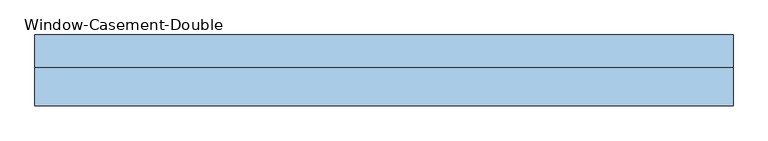
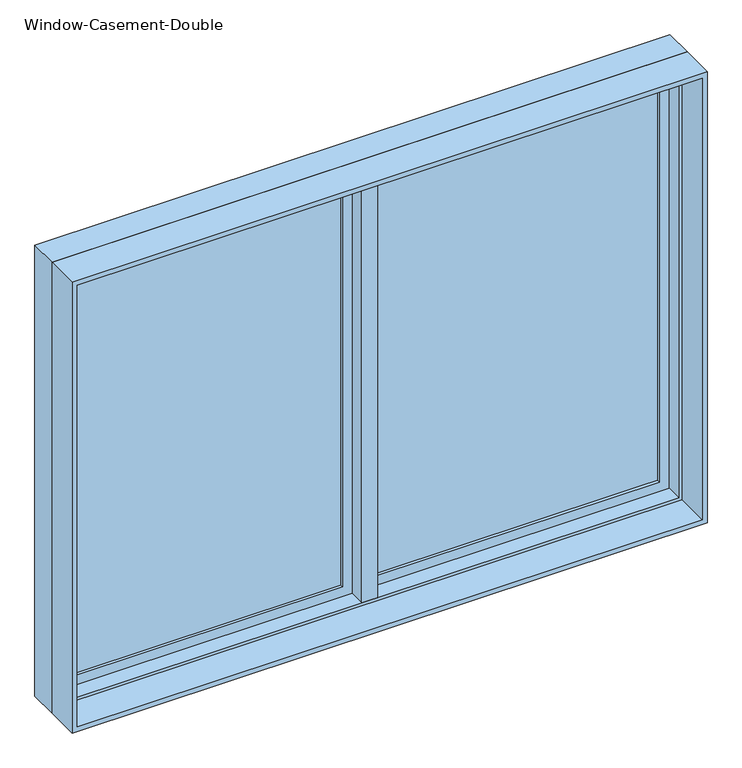
"""IFC4 building model written with IfcOpenShell, lengths in millimetres: window geometry, Window-Casement-Double."""

from ifc_helpers import new_model, si_unit, frame, origin, place, context, project, spatial, polyline, outline, extrude, faceted_brep, source, transform, mapped, element, save


def window_casement_double_9ae172a2(model_context):
    return source(origin(), model_context, "Body", "SolidModel", [
        faceted_brep([(9.525, 133.35, 2730.5), (-9.525, 133.35, 2730.5), (-9.525, 82.55, 2730.5), (9.525, 82.55, 2730.5), (9.525, 133.35, 927.1), (9.525, 82.55, 927.1), (-9.525, 82.55, 927.1), (-9.525, 133.35, 927.1), (-9.525, 82.55, 946.15), (-9.525, 82.55, 2711.45), (-30.1625, 82.55, 946.15), (-30.1625, 82.55, 2711.45), (-30.1625, 19.05, 946.15), (-30.1625, 19.05, 2711.45), (30.1625, 19.05, 946.15), (30.1625, 19.05, 2711.45), (30.1625, 82.55, 946.15), (30.1625, 82.55, 2711.45), (9.525, 82.55, 946.15), (9.525, 82.55, 2711.45)], [[[0, 1, 2, 3]], [[4, 5, 6, 7]], [[1, 0, 4, 7]], [[2, 1, 7, 6, 8, 9]], [[9, 8, 10, 11]], [[11, 10, 12, 13]], [[13, 12, 14, 15]], [[15, 14, 16, 17]], [[17, 16, 18, 19]], [[0, 3, 19, 18, 5, 4]], [[18, 8, 6, 5]], [[9, 19, 3, 2]], [[8, 18, 16, 14, 12, 10]], [[19, 9, 11, 13, 15, 17]]]),
        extrude(outline(polyline([(-66.675, 114.3), (-66.675, 107.95), (-1149.35, 107.95), (-1149.35, 114.3), (-66.675, 114.3)])), frame((0.0, 0.0, 984.25), z_axis=(0.0, 0.0, 1.0), x_axis=(1.0, 0.0, 0.0)), (0.0, 0.0, 1.0), 1689.1),
        extrude(outline(polyline([(-1149.35, 95.25), (-1149.35, 101.6), (-66.675, 101.6), (-66.675, 95.25), (-1149.35, 95.25)])), frame((0.0, 0.0, 984.25), z_axis=(0.0, 0.0, 1.0), x_axis=(1.0, 0.0, 0.0)), (0.0, 0.0, 1.0), 1689.1),
        extrude(outline(polyline([(1149.35, 114.3), (1149.35, 107.95), (66.675, 107.95), (66.675, 114.3), (1149.35, 114.3)])), frame((0.0, 0.0, 984.25), z_axis=(0.0, 0.0, 1.0), x_axis=(1.0, 0.0, 0.0)), (0.0, 0.0, 1.0), 1689.1),
        extrude(outline(polyline([(66.675, 95.25), (66.675, 101.6), (1149.35, 101.6), (1149.35, 95.25), (66.675, 95.25)])), frame((0.0, 0.0, 984.25), z_axis=(0.0, 0.0, 1.0), x_axis=(1.0, 0.0, 0.0)), (0.0, 0.0, 1.0), 1689.1),
        extrude(outline(polyline([(2730.5, -1206.5), (927.1, -1206.5), (927.1, -9.525), (2730.5, -9.525), (2730.5, -1206.5)]), holes=[polyline([(2673.35, -66.675), (984.25, -66.675), (984.25, -1149.35), (2673.35, -1149.35), (2673.35, -66.675)])]), frame((0.0, 82.55, 0.0), z_axis=(0.0, 1.0, 0.0), x_axis=(0.0, 0.0, 1.0)), (0.0, 0.0, 1.0), 44.45),
        extrude(outline(polyline([(927.1, 1206.5), (2730.5, 1206.5), (2730.5, 9.525), (927.1, 9.525), (927.1, 1206.5)]), holes=[polyline([(984.25, 66.675), (2673.35, 66.675), (2673.35, 1149.35), (984.25, 1149.35), (984.25, 66.675)])]), frame((0.0, 82.55, 0.0), z_axis=(0.0, 1.0, 0.0), x_axis=(0.0, 0.0, 1.0)), (0.0, 0.0, 1.0), 44.45),
        extrude(outline(polyline([(2743.2, -1219.2), (914.4, -1219.2), (914.4, 1219.2), (2743.2, 1219.2), (2743.2, -1219.2)]), holes=[polyline([(2724.15, 1200.15), (933.45, 1200.15), (933.45, -1200.15), (2724.15, -1200.15), (2724.15, 1200.15)])]), frame((0.0, -114.3, 0.0), z_axis=(0.0, 1.0, 0.0), x_axis=(0.0, 0.0, 1.0)), (0.0, 0.0, 1.0), 133.35),
        faceted_brep([(1187.45, 82.55, 2711.45), (1187.45, 19.05, 2711.45), (-1187.45, 19.05, 2711.45), (-1187.45, 82.55, 2711.45), (1206.5, 133.35, 2730.5), (1206.5, 82.55, 2730.5), (-1206.5, 82.55, 2730.5), (-1206.5, 133.35, 2730.5), (1219.2, 19.05, 2743.2), (1219.2, 133.35, 2743.2), (-1219.2, 133.35, 2743.2), (-1219.2, 19.05, 2743.2), (-1187.45, 19.05, 946.15), (-1187.45, 82.55, 946.15), (-1206.5, 82.55, 927.1), (-1206.5, 133.35, 927.1), (-1219.2, 133.35, 914.4), (-1219.2, 19.05, 914.4), (1187.45, 19.05, 946.15), (1187.45, 82.55, 946.15), (1206.5, 82.55, 927.1), (1206.5, 133.35, 927.1), (1219.2, 133.35, 914.4), (1219.2, 19.05, 914.4)], [[[0, 1, 2, 3]], [[4, 5, 6, 7]], [[8, 9, 10, 11]], [[3, 2, 12, 13]], [[7, 6, 14, 15]], [[11, 10, 16, 17]], [[13, 12, 18, 19]], [[15, 14, 20, 21]], [[17, 16, 22, 23]], [[11, 17, 23, 8], [1, 18, 12, 2]], [[19, 18, 1, 0]], [[5, 20, 14, 6], [3, 13, 19, 0]], [[21, 20, 5, 4]], [[23, 22, 9, 8]], [[9, 22, 16, 10], [7, 15, 21, 4]]]),
    ])


if __name__ == "__main__":
    model = new_model("IFC4")
    model_context = context("Model", 3, world=origin())
    ifc_project = project(units=[si_unit("LENGTHUNIT", "METRE", prefix="MILLI")], contexts=[model_context])
    site = spatial("IfcSite", under=ifc_project)
    building = spatial("IfcBuilding", under=site)
    placement = place(None, origin())
    window_casement_double_shape = window_casement_double_9ae172a2(model_context)
    element("IfcWindow", 1, ObjectType="Window-Casement-Double", at=placement, inside=building, context=model_context, shape_type="MappedRepresentation", body=[
        mapped(window_casement_double_shape, transform((0.0, 0.0, 0.0), x_axis=(1.0, 0.0, 0.0), y_axis=(0.0, 1.0, 0.0), z_axis=(0.0, 0.0, 1.0))),
    ])
    save(model, "model.ifc")

# Revit data of these elements
# Type "Window-Casement-Double"
#   Type Mark = "19"
#   Fire Rating = "0.5h"
#   Assembly Code = "B2020100"
#   Analytic Construction = "Double glazing - domestic"
#   Frame Extension [instance default] = 0' - 0 1/4"
#   Window Inset [instance default] = 0' - 0"
#   Wall Thickness [instance default] = 0' - 6"
#   Interior Wall Closure [instance default] = 0' - 2 1/4"
#   Half Width = 4' - 0"
#   Visual Light Transmittance = 0.81
#   Thermal Resistance (R) = 1.8146 (h·ft²·°F)/BTU
#   Solar Heat Gain Coefficient = 0.76
#   Rough Width = 8' - 0 1/2"
#   Rough Height = 6' - 0 1/2"
#   Height = 6' - 0"
#   Heat Transfer Coefficient (U) = 0.5511 BTU/(h·ft²·°F)
#   Exterior Wall Closure [instance default] = 0' - 1 1/4"
#   Extension Jamb [instance default] = 0' - 2 1/4"
#   Default Sill Height = 3' - 0"
#   Width = 8' - 0"
#   Muntin Visibility = yes
#   Interior Trim Visibility [instance default] = yes
#   Exterior Trim Visibility [instance default] = yes
#   Extension Jamb Visibility [instance default] = yes
#   Interior Trim Material = Wood - Stained
#   Muntin Pattern = Muntin Pattern_2x2 : Muntin Pattern_2x2
#   Interior Trim = Trim-Window-Interior-Flat : Picture Frame
#   Interior Frame Material = Wood - Stained
#   Glass Panel Material = Glass
#   Exterior Trim Material = Clad - White
#   Exterior Trim = Trim-Window-Exterior-Flat : with Sill
#   Exterior Frame Material = Clad - White
#   Wall Closure = (empty or 0)
# Element 1 (IfcWindow, "Window-Casement-Double")
#   Wall Thickness = 0' - 9"
#   Extension Jamb = 0' - 5 1/4"
#   Materials on its faces: "Wood - Stained", "Glass", "Clad - White"
# Materials
#   "Wood - Stained": class "Wood", colour RGB 224 178 126, transparency 0, Cost = 0
#   "Glass": class "Glass", colour RGB 0 128 192, transparency 0.75, Description = "Soda Lime Glass", Cost = 0
#   "Clad - White": class "Wood", colour RGB 242 242 238, transparency 0, Cost = 0
